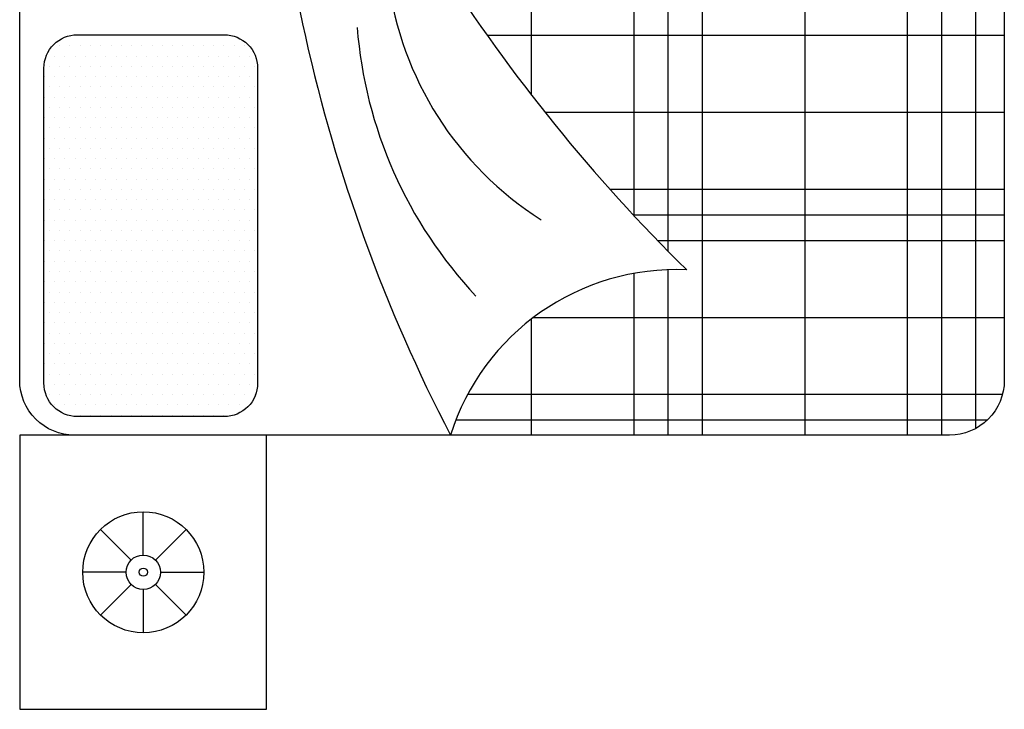
# Model space of a CAD drawing. Units: inches. Extents: x 528 to 2520, y -151 to 1354.
# Tile 32 of 41: x 2171 to 2226, y 731 to 770. Entities that reach past the tile are written whole.
import ezdxf

# ---------------------------------------------------------------- set-up
doc = ezdxf.new("R2010")
doc.units = ezdxf.units.IN
doc.header["$MEASUREMENT"] = 0
doc.layers.add('A-FURN', color=8, linetype='Continuous', lineweight=18)
doc.layers.add('BLOCK', color=6, linetype='Continuous')

# ---------------------------------------------------------------- blocks, each defined once
blk = doc.blocks.new('*X15')
at = {"color": 0}
for p, q in [((276.598, 451.25), (280.51, 451.25)), ((275.455, 450.625), (280.51, 450.625)), ((274.411, 450), (280.51, 450)), ((265.51, 448.125), (267.634, 448.125)), ((271.723, 448.125), (280.51, 448.125)), ((265.51, 446.25), (268.465, 446.25)), ((269.519, 446.25), (280.51, 446.25)), ((265.51, 445.625), (268.531, 445.625)), ((268.866, 445.625), (280.51, 445.625)), ((265.51, 445), (280.51, 445)), ((265.51, 443.125), (280.51, 443.125)), ((265.51, 441.25), (280.51, 441.25)), ((265.51, 440.625), (280.51, 440.625)), ((265.634, 440), (280.386, 440))]:
    blk.add_line(p, q, dxfattribs=at)
blk = doc.blocks.new('*X16')
at = {"color": 0}
for p, q in [((280.312, 439.886), (280.312, 452.896)), ((278.906, 439.482), (278.906, 452.338)), ((277.5, 439.482), (277.5, 451.702)), ((277.031, 439.482), (277.031, 451.471)), ((276.562, 439.482), (276.562, 451.231)), ((275.156, 439.482), (275.156, 450.451)), ((265.781, 439.797), (265.781, 449.511)), ((273.75, 439.482), (273.75, 449.576)), ((266.25, 439.517), (266.25, 449.296)), ((273.281, 439.482), (273.281, 449.261)), ((272.812, 439.482), (272.812, 448.934)), ((267.656, 439.482), (267.656, 448.095)), ((271.406, 439.482), (271.406, 447.876)), ((270, 439.482), (270, 446.689)), ((269.531, 439.482), (269.531, 446.262)), ((269.062, 439.482), (269.062, 445.817))]:
    blk.add_line(p, q, dxfattribs=at)
blk = doc.blocks.new('*X17')
at = {"color": 0}
for p, q in [((266.4375, 457.03125), (266.4375, 457.03125)), ((266.8125, 457.03125), (266.8125, 457.03125)), ((267.1875, 457.03125), (267.1875, 457.03125)), ((267.5625, 457.03125), (267.5625, 457.03125)), ((267.9375, 457.03125), (267.9375, 457.03125)), ((268.3125, 457.03125), (268.3125, 457.03125)), ((268.6875, 457.03125), (268.6875, 457.03125)), ((269.0625, 457.03125), (269.0625, 457.03125)), ((269.4375, 457.03125), (269.4375, 457.03125)), ((269.8125, 457.03125), (269.8125, 457.03125)), ((270.1875, 457.03125), (270.1875, 457.03125)), ((270.5625, 457.03125), (270.5625, 457.03125)), ((270.9375, 457.03125), (270.9375, 457.03125)), ((271.3125, 457.03125), (271.3125, 457.03125)), ((271.6875, 457.03125), (271.6875, 457.03125)), ((272.0625, 457.03125), (272.0625, 457.03125)), ((266.0625, 456.84375), (266.0625, 456.84375)), ((266.25, 456.9375), (266.25, 456.9375)), ((266.4375, 456.84375), (266.4375, 456.84375)), ((266.625, 456.9375), (266.625, 456.9375)), ((266.8125, 456.84375), (266.8125, 456.84375)), ((267, 456.9375), (267, 456.9375)), ((267.1875, 456.84375), (267.1875, 456.84375)), ((267.375, 456.9375), (267.375, 456.9375)), ((267.5625, 456.84375), (267.5625, 456.84375)), ((267.75, 456.9375), (267.75, 456.9375)), ((267.9375, 456.84375), (267.9375, 456.84375)), ((268.125, 456.9375), (268.125, 456.9375)), ((268.3125, 456.84375), (268.3125, 456.84375)), ((268.5, 456.9375), (268.5, 456.9375)), ((268.6875, 456.84375), (268.6875, 456.84375)), ((268.875, 456.9375), (268.875, 456.9375)), ((269.0625, 456.84375), (269.0625, 456.84375)), ((269.25, 456.9375), (269.25, 456.9375)), ((269.4375, 456.84375), (269.4375, 456.84375)), ((269.625, 456.9375), (269.625, 456.9375)), ((269.8125, 456.84375), (269.8125, 456.84375)), ((270, 456.9375), (270, 456.9375)), ((270.1875, 456.84375), (270.1875, 456.84375)), ((270.375, 456.9375), (270.375, 456.9375)), ((270.5625, 456.84375), (270.5625, 456.84375)), ((270.75, 456.9375), (270.75, 456.9375)), ((270.9375, 456.84375), (270.9375, 456.84375)), ((271.125, 456.9375), (271.125, 456.9375)), ((271.3125, 456.84375), (271.3125, 456.84375)), ((271.5, 456.9375), (271.5, 456.9375)), ((271.6875, 456.84375), (271.6875, 456.84375)), ((271.875, 456.9375), (271.875, 456.9375)), ((272.0625, 456.84375), (272.0625, 456.84375)), ((272.25, 456.9375), (272.25, 456.9375)), ((272.4375, 456.84375), (272.4375, 456.84375)), ((266.25, 456.75), (266.25, 456.75)), ((266.625, 456.75), (266.625, 456.75)), ((267, 456.75), (267, 456.75)), ((267.375, 456.75), (267.375, 456.75)), ((267.75, 456.75), (267.75, 456.75)), ((268.125, 456.75), (268.125, 456.75)), ((268.5, 456.75), (268.5, 456.75)), ((268.875, 456.75), (268.875, 456.75)), ((269.25, 456.75), (269.25, 456.75)), ((269.625, 456.75), (269.625, 456.75)), ((270, 456.75), (270, 456.75)), ((270.375, 456.75), (270.375, 456.75)), ((270.75, 456.75), (270.75, 456.75)), ((271.125, 456.75), (271.125, 456.75)), ((271.5, 456.75), (271.5, 456.75)), ((271.875, 456.75), (271.875, 456.75)), ((272.25, 456.75), (272.25, 456.75)), ((272.625, 456.75), (272.625, 456.75)), ((265.875, 456.5625), (265.875, 456.5625)), ((266.0625, 456.65625), (266.0625, 456.65625)), ((266.25, 456.5625), (266.25, 456.5625)), ((266.4375, 456.65625), (266.4375, 456.65625)), ((266.625, 456.5625), (266.625, 456.5625)), ((266.8125, 456.65625), (266.8125, 456.65625)), ((267, 456.5625), (267, 456.5625)), ((267.1875, 456.65625), (267.1875, 456.65625)), ((267.375, 456.5625), (267.375, 456.5625)), ((267.5625, 456.65625), (267.5625, 456.65625)), ((267.75, 456.5625), (267.75, 456.5625)), ((267.9375, 456.65625), (267.9375, 456.65625)), ((268.125, 456.5625), (268.125, 456.5625)), ((268.3125, 456.65625), (268.3125, 456.65625)), ((268.5, 456.5625), (268.5, 456.5625)), ((268.6875, 456.65625), (268.6875, 456.65625)), ((268.875, 456.5625), (268.875, 456.5625)), ((269.0625, 456.65625), (269.0625, 456.65625)), ((269.25, 456.5625), (269.25, 456.5625)), ((269.4375, 456.65625), (269.4375, 456.65625)), ((269.625, 456.5625), (269.625, 456.5625)), ((269.8125, 456.65625), (269.8125, 456.65625)), ((270, 456.5625), (270, 456.5625)), ((270.1875, 456.65625), (270.1875, 456.65625)), ((270.375, 456.5625), (270.375, 456.5625)), ((270.5625, 456.65625), (270.5625, 456.65625)), ((270.75, 456.5625), (270.75, 456.5625)), ((270.9375, 456.65625), (270.9375, 456.65625)), ((271.125, 456.5625), (271.125, 456.5625)), ((271.3125, 456.65625), (271.3125, 456.65625)), ((271.5, 456.5625), (271.5, 456.5625)), ((271.6875, 456.65625), (271.6875, 456.65625)), ((271.875, 456.5625), (271.875, 456.5625)), ((272.0625, 456.65625), (272.0625, 456.65625)), ((272.25, 456.5625), (272.25, 456.5625)), ((272.4375, 456.65625), (272.4375, 456.65625)), ((272.625, 456.5625), (272.625, 456.5625)), ((265.875, 456.375), (265.875, 456.375)), ((266.0625, 456.46875), (266.0625, 456.46875)), ((266.25, 456.375), (266.25, 456.375)), ((266.4375, 456.46875), (266.4375, 456.46875)), ((266.625, 456.375), (266.625, 456.375)), ((266.8125, 456.46875), (266.8125, 456.46875)), ((267, 456.375), (267, 456.375)), ((267.1875, 456.46875), (267.1875, 456.46875)), ((267.375, 456.375), (267.375, 456.375)), ((267.5625, 456.46875), (267.5625, 456.46875)), ((267.75, 456.375), (267.75, 456.375)), ((267.9375, 456.46875), (267.9375, 456.46875)), ((268.125, 456.375), (268.125, 456.375)), ((268.3125, 456.46875), (268.3125, 456.46875)), ((268.5, 456.375), (268.5, 456.375)), ((268.6875, 456.46875), (268.6875, 456.46875)), ((268.875, 456.375), (268.875, 456.375)), ((269.0625, 456.46875), (269.0625, 456.46875)), ((269.25, 456.375), (269.25, 456.375)), ((269.4375, 456.46875), (269.4375, 456.46875)), ((269.625, 456.375), (269.625, 456.375)), ((269.8125, 456.46875), (269.8125, 456.46875)), ((270, 456.375), (270, 456.375)), ((270.1875, 456.46875), (270.1875, 456.46875)), ((270.375, 456.375), (270.375, 456.375)), ((270.5625, 456.46875), (270.5625, 456.46875)), ((270.75, 456.375), (270.75, 456.375)), ((270.9375, 456.46875), (270.9375, 456.46875)), ((271.125, 456.375), (271.125, 456.375)), ((271.3125, 456.46875), (271.3125, 456.46875)), ((271.5, 456.375), (271.5, 456.375)), ((271.6875, 456.46875), (271.6875, 456.46875)), ((271.875, 456.375), (271.875, 456.375)), ((272.0625, 456.46875), (272.0625, 456.46875)), ((272.25, 456.375), (272.25, 456.375)), ((272.4375, 456.46875), (272.4375, 456.46875)), ((272.625, 456.375), (272.625, 456.375)), ((272.8125, 456.46875), (272.8125, 456.46875)), ((265.875, 456.1875), (265.875, 456.1875)), ((266.0625, 456.28125), (266.0625, 456.28125)), ((266.25, 456.1875), (266.25, 456.1875)), ((266.4375, 456.28125), (266.4375, 456.28125)), ((266.625, 456.1875), (266.625, 456.1875)), ((266.8125, 456.28125), (266.8125, 456.28125)), ((267, 456.1875), (267, 456.1875)), ((267.1875, 456.28125), (267.1875, 456.28125)), ((267.375, 456.1875), (267.375, 456.1875)), ((267.5625, 456.28125), (267.5625, 456.28125)), ((267.75, 456.1875), (267.75, 456.1875)), ((267.9375, 456.28125), (267.9375, 456.28125)), ((268.125, 456.1875), (268.125, 456.1875)), ((268.3125, 456.28125), (268.3125, 456.28125)), ((268.5, 456.1875), (268.5, 456.1875)), ((268.6875, 456.28125), (268.6875, 456.28125)), ((268.875, 456.1875), (268.875, 456.1875)), ((269.0625, 456.28125), (269.0625, 456.28125)), ((269.25, 456.1875), (269.25, 456.1875)), ((269.4375, 456.28125), (269.4375, 456.28125)), ((269.625, 456.1875), (269.625, 456.1875)), ((269.8125, 456.28125), (269.8125, 456.28125)), ((270, 456.1875), (270, 456.1875)), ((270.1875, 456.28125), (270.1875, 456.28125)), ((270.375, 456.1875), (270.375, 456.1875)), ((270.5625, 456.28125), (270.5625, 456.28125)), ((270.75, 456.1875), (270.75, 456.1875)), ((270.9375, 456.28125), (270.9375, 456.28125)), ((271.125, 456.1875), (271.125, 456.1875)), ((271.3125, 456.28125), (271.3125, 456.28125)), ((271.5, 456.1875), (271.5, 456.1875)), ((271.6875, 456.28125), (271.6875, 456.28125)), ((271.875, 456.1875), (271.875, 456.1875)), ((272.0625, 456.28125), (272.0625, 456.28125)), ((272.25, 456.1875), (272.25, 456.1875)), ((272.4375, 456.28125), (272.4375, 456.28125)), ((272.625, 456.1875), (272.625, 456.1875)), ((272.8125, 456.28125), (272.8125, 456.28125)), ((265.875, 456), (265.875, 456)), ((266.0625, 456.09375), (266.0625, 456.09375)), ((266.25, 456), (266.25, 456)), ((266.4375, 456.09375), (266.4375, 456.09375)), ((266.625, 456), (266.625, 456)), ((266.8125, 456.09375), (266.8125, 456.09375)), ((267, 456), (267, 456)), ((267.1875, 456.09375), (267.1875, 456.09375)), ((267.375, 456), (267.375, 456)), ((267.5625, 456.09375), (267.5625, 456.09375)), ((267.75, 456), (267.75, 456)), ((267.9375, 456.09375), (267.9375, 456.09375)), ((268.125, 456), (268.125, 456)), ((268.3125, 456.09375), (268.3125, 456.09375)), ((268.5, 456), (268.5, 456)), ((268.6875, 456.09375), (268.6875, 456.09375)), ((268.875, 456), (268.875, 456)), ((269.0625, 456.09375), (269.0625, 456.09375)), ((269.25, 456), (269.25, 456)), ((269.4375, 456.09375), (269.4375, 456.09375)), ((269.625, 456), (269.625, 456)), ((269.8125, 456.09375), (269.8125, 456.09375)), ((270, 456), (270, 456)), ((270.1875, 456.09375), (270.1875, 456.09375)), ((270.375, 456), (270.375, 456)), ((270.5625, 456.09375), (270.5625, 456.09375)), ((270.75, 456), (270.75, 456)), ((270.9375, 456.09375), (270.9375, 456.09375)), ((271.125, 456), (271.125, 456)), ((271.3125, 456.09375), (271.3125, 456.09375)), ((271.5, 456), (271.5, 456)), ((271.6875, 456.09375), (271.6875, 456.09375)), ((271.875, 456), (271.875, 456)), ((272.0625, 456.09375), (272.0625, 456.09375)), ((272.25, 456), (272.25, 456)), ((272.4375, 456.09375), (272.4375, 456.09375)), ((272.625, 456), (272.625, 456)), ((272.8125, 456.09375), (272.8125, 456.09375)), ((265.875, 455.8125), (265.875, 455.8125)), ((266.0625, 455.90625), (266.0625, 455.90625)), ((266.25, 455.8125), (266.25, 455.8125)), ((266.4375, 455.90625), (266.4375, 455.90625)), ((266.625, 455.8125), (266.625, 455.8125)), ((266.8125, 455.90625), (266.8125, 455.90625)), ((267, 455.8125), (267, 455.8125)), ((267.1875, 455.90625), (267.1875, 455.90625)), ((267.375, 455.8125), (267.375, 455.8125)), ((267.5625, 455.90625), (267.5625, 455.90625)), ((267.75, 455.8125), (267.75, 455.8125)), ((267.9375, 455.90625), (267.9375, 455.90625)), ((268.125, 455.8125), (268.125, 455.8125)), ((268.3125, 455.90625), (268.3125, 455.90625)), ((268.5, 455.8125), (268.5, 455.8125)), ((268.6875, 455.90625), (268.6875, 455.90625)), ((268.875, 455.8125), (268.875, 455.8125)), ((269.0625, 455.90625), (269.0625, 455.90625)), ((269.25, 455.8125), (269.25, 455.8125)), ((269.4375, 455.90625), (269.4375, 455.90625)), ((269.625, 455.8125), (269.625, 455.8125)), ((269.8125, 455.90625), (269.8125, 455.90625)), ((270, 455.8125), (270, 455.8125)), ((270.1875, 455.90625), (270.1875, 455.90625)), ((270.375, 455.8125), (270.375, 455.8125)), ((270.5625, 455.90625), (270.5625, 455.90625)), ((270.75, 455.8125), (270.75, 455.8125)), ((270.9375, 455.90625), (270.9375, 455.90625)), ((271.125, 455.8125), (271.125, 455.8125)), ((271.3125, 455.90625), (271.3125, 455.90625)), ((271.5, 455.8125), (271.5, 455.8125)), ((271.6875, 455.90625), (271.6875, 455.90625)), ((271.875, 455.8125), (271.875, 455.8125)), ((272.0625, 455.90625), (272.0625, 455.90625)), ((272.25, 455.8125), (272.25, 455.8125)), ((272.4375, 455.90625), (272.4375, 455.90625)), ((272.625, 455.8125), (272.625, 455.8125)), ((272.8125, 455.90625), (272.8125, 455.90625)), ((265.875, 455.625), (265.875, 455.625)), ((266.0625, 455.71875), (266.0625, 455.71875)), ((266.25, 455.625), (266.25, 455.625)), ((266.4375, 455.71875), (266.4375, 455.71875)), ((266.625, 455.625), (266.625, 455.625)), ((266.8125, 455.71875), (266.8125, 455.71875)), ((267, 455.625), (267, 455.625)), ((267.1875, 455.71875), (267.1875, 455.71875)), ((267.375, 455.625), (267.375, 455.625)), ((267.5625, 455.71875), (267.5625, 455.71875)), ((267.75, 455.625), (267.75, 455.625)), ((267.9375, 455.71875), (267.9375, 455.71875)), ((268.125, 455.625), (268.125, 455.625)), ((268.3125, 455.71875), (268.3125, 455.71875)), ((268.5, 455.625), (268.5, 455.625)), ((268.6875, 455.71875), (268.6875, 455.71875)), ((268.875, 455.625), (268.875, 455.625)), ((269.0625, 455.71875), (269.0625, 455.71875)), ((269.25, 455.625), (269.25, 455.625)), ((269.4375, 455.71875), (269.4375, 455.71875)), ((269.625, 455.625), (269.625, 455.625)), ((269.8125, 455.71875), (269.8125, 455.71875)), ((270, 455.625), (270, 455.625)), ((270.1875, 455.71875), (270.1875, 455.71875)), ((270.375, 455.625), (270.375, 455.625)), ((270.5625, 455.71875), (270.5625, 455.71875)), ((270.75, 455.625), (270.75, 455.625)), ((270.9375, 455.71875), (270.9375, 455.71875)), ((271.125, 455.625), (271.125, 455.625)), ((271.3125, 455.71875), (271.3125, 455.71875)), ((271.5, 455.625), (271.5, 455.625)), ((271.6875, 455.71875), (271.6875, 455.71875)), ((271.875, 455.625), (271.875, 455.625)), ((272.0625, 455.71875), (272.0625, 455.71875)), ((272.25, 455.625), (272.25, 455.625)), ((272.4375, 455.71875), (272.4375, 455.71875)), ((272.625, 455.625), (272.625, 455.625)), ((272.8125, 455.71875), (272.8125, 455.71875)), ((265.875, 455.4375), (265.875, 455.4375)), ((266.0625, 455.53125), (266.0625, 455.53125)), ((266.25, 455.4375), (266.25, 455.4375)), ((266.4375, 455.53125), (266.4375, 455.53125)), ((266.625, 455.4375), (266.625, 455.4375)), ((266.8125, 455.53125), (266.8125, 455.53125)), ((267, 455.4375), (267, 455.4375)), ((267.1875, 455.53125), (267.1875, 455.53125)), ((267.375, 455.4375), (267.375, 455.4375)), ((267.5625, 455.53125), (267.5625, 455.53125)), ((267.75, 455.4375), (267.75, 455.4375)), ((267.9375, 455.53125), (267.9375, 455.53125)), ((268.125, 455.4375), (268.125, 455.4375)), ((268.3125, 455.53125), (268.3125, 455.53125)), ((268.5, 455.4375), (268.5, 455.4375)), ((268.6875, 455.53125), (268.6875, 455.53125)), ((268.875, 455.4375), (268.875, 455.4375)), ((269.0625, 455.53125), (269.0625, 455.53125)), ((269.25, 455.4375), (269.25, 455.4375)), ((269.4375, 455.53125), (269.4375, 455.53125)), ((269.625, 455.4375), (269.625, 455.4375)), ((269.8125, 455.53125), (269.8125, 455.53125)), ((270, 455.4375), (270, 455.4375)), ((270.1875, 455.53125), (270.1875, 455.53125)), ((270.375, 455.4375), (270.375, 455.4375)), ((270.5625, 455.53125), (270.5625, 455.53125)), ((270.75, 455.4375), (270.75, 455.4375)), ((270.9375, 455.53125), (270.9375, 455.53125)), ((271.125, 455.4375), (271.125, 455.4375)), ((271.3125, 455.53125), (271.3125, 455.53125)), ((271.5, 455.4375), (271.5, 455.4375)), ((271.6875, 455.53125), (271.6875, 455.53125)), ((271.875, 455.4375), (271.875, 455.4375)), ((272.0625, 455.53125), (272.0625, 455.53125)), ((272.25, 455.4375), (272.25, 455.4375)), ((272.4375, 455.53125), (272.4375, 455.53125)), ((272.625, 455.4375), (272.625, 455.4375)), ((272.8125, 455.53125), (272.8125, 455.53125)), ((265.875, 455.25), (265.875, 455.25)), ((266.0625, 455.34375), (266.0625, 455.34375)), ((266.25, 455.25), (266.25, 455.25)), ((266.4375, 455.34375), (266.4375, 455.34375)), ((266.625, 455.25), (266.625, 455.25)), ((266.8125, 455.34375), (266.8125, 455.34375)), ((267, 455.25), (267, 455.25)), ((267.1875, 455.34375), (267.1875, 455.34375)), ((267.375, 455.25), (267.375, 455.25)), ((267.5625, 455.34375), (267.5625, 455.34375)), ((267.75, 455.25), (267.75, 455.25)), ((267.9375, 455.34375), (267.9375, 455.34375)), ((268.125, 455.25), (268.125, 455.25)), ((268.3125, 455.34375), (268.3125, 455.34375)), ((268.5, 455.25), (268.5, 455.25)), ((268.6875, 455.34375), (268.6875, 455.34375)), ((268.875, 455.25), (268.875, 455.25)), ((269.0625, 455.34375), (269.0625, 455.34375)), ((269.25, 455.25), (269.25, 455.25)), ((269.4375, 455.34375), (269.4375, 455.34375)), ((269.625, 455.25), (269.625, 455.25)), ((269.8125, 455.34375), (269.8125, 455.34375)), ((270, 455.25), (270, 455.25)), ((270.1875, 455.34375), (270.1875, 455.34375)), ((270.375, 455.25), (270.375, 455.25)), ((270.5625, 455.34375), (270.5625, 455.34375)), ((270.75, 455.25), (270.75, 455.25)), ((270.9375, 455.34375), (270.9375, 455.34375)), ((271.125, 455.25), (271.125, 455.25)), ((271.3125, 455.34375), (271.3125, 455.34375)), ((271.5, 455.25), (271.5, 455.25)), ((271.6875, 455.34375), (271.6875, 455.34375)), ((271.875, 455.25), (271.875, 455.25)), ((272.0625, 455.34375), (272.0625, 455.34375)), ((272.25, 455.25), (272.25, 455.25)), ((272.4375, 455.34375), (272.4375, 455.34375)), ((272.625, 455.25), (272.625, 455.25)), ((272.8125, 455.34375), (272.8125, 455.34375)), ((265.875, 455.0625), (265.875, 455.0625)), ((266.0625, 455.15625), (266.0625, 455.15625)), ((266.25, 455.0625), (266.25, 455.0625)), ((266.4375, 455.15625), (266.4375, 455.15625)), ((266.625, 455.0625), (266.625, 455.0625)), ((266.8125, 455.15625), (266.8125, 455.15625)), ((267, 455.0625), (267, 455.0625)), ((267.1875, 455.15625), (267.1875, 455.15625)), ((267.375, 455.0625), (267.375, 455.0625)), ((267.5625, 455.15625), (267.5625, 455.15625)), ((267.75, 455.0625), (267.75, 455.0625)), ((267.9375, 455.15625), (267.9375, 455.15625)), ((268.125, 455.0625), (268.125, 455.0625)), ((268.3125, 455.15625), (268.3125, 455.15625)), ((268.5, 455.0625), (268.5, 455.0625)), ((268.6875, 455.15625), (268.6875, 455.15625)), ((268.875, 455.0625), (268.875, 455.0625)), ((269.0625, 455.15625), (269.0625, 455.15625)), ((269.25, 455.0625), (269.25, 455.0625)), ((269.4375, 455.15625), (269.4375, 455.15625)), ((269.625, 455.0625), (269.625, 455.0625)), ((269.8125, 455.15625), (269.8125, 455.15625)), ((270, 455.0625), (270, 455.0625)), ((270.1875, 455.15625), (270.1875, 455.15625)), ((270.375, 455.0625), (270.375, 455.0625)), ((270.5625, 455.15625), (270.5625, 455.15625)), ((270.75, 455.0625), (270.75, 455.0625)), ((270.9375, 455.15625), (270.9375, 455.15625)), ((271.125, 455.0625), (271.125, 455.0625)), ((271.3125, 455.15625), (271.3125, 455.15625)), ((271.5, 455.0625), (271.5, 455.0625)), ((271.6875, 455.15625), (271.6875, 455.15625)), ((271.875, 455.0625), (271.875, 455.0625)), ((272.0625, 455.15625), (272.0625, 455.15625)), ((272.25, 455.0625), (272.25, 455.0625)), ((272.4375, 455.15625), (272.4375, 455.15625)), ((272.625, 455.0625), (272.625, 455.0625)), ((272.8125, 455.15625), (272.8125, 455.15625)), ((265.875, 454.875), (265.875, 454.875)), ((266.0625, 454.96875), (266.0625, 454.96875)), ((266.25, 454.875), (266.25, 454.875)), ((266.4375, 454.96875), (266.4375, 454.96875)), ((266.625, 454.875), (266.625, 454.875)), ((266.8125, 454.96875), (266.8125, 454.96875)), ((267, 454.875), (267, 454.875)), ((267.1875, 454.96875), (267.1875, 454.96875)), ((267.375, 454.875), (267.375, 454.875)), ((267.5625, 454.96875), (267.5625, 454.96875)), ((267.75, 454.875), (267.75, 454.875)), ((267.9375, 454.96875), (267.9375, 454.96875)), ((268.125, 454.875), (268.125, 454.875)), ((268.3125, 454.96875), (268.3125, 454.96875)), ((268.5, 454.875), (268.5, 454.875)), ((268.6875, 454.96875), (268.6875, 454.96875)), ((268.875, 454.875), (268.875, 454.875)), ((269.0625, 454.96875), (269.0625, 454.96875)), ((269.25, 454.875), (269.25, 454.875)), ((269.4375, 454.96875), (269.4375, 454.96875)), ((269.625, 454.875), (269.625, 454.875)), ((269.8125, 454.96875), (269.8125, 454.96875)), ((270, 454.875), (270, 454.875)), ((270.1875, 454.96875), (270.1875, 454.96875)), ((270.375, 454.875), (270.375, 454.875)), ((270.5625, 454.96875), (270.5625, 454.96875)), ((270.75, 454.875), (270.75, 454.875)), ((270.9375, 454.96875), (270.9375, 454.96875)), ((271.125, 454.875), (271.125, 454.875)), ((271.3125, 454.96875), (271.3125, 454.96875)), ((271.5, 454.875), (271.5, 454.875)), ((271.6875, 454.96875), (271.6875, 454.96875)), ((271.875, 454.875), (271.875, 454.875)), ((272.0625, 454.96875), (272.0625, 454.96875)), ((272.25, 454.875), (272.25, 454.875)), ((272.4375, 454.96875), (272.4375, 454.96875)), ((272.625, 454.875), (272.625, 454.875)), ((272.8125, 454.96875), (272.8125, 454.96875)), ((265.875, 454.6875), (265.875, 454.6875)), ((266.0625, 454.78125), (266.0625, 454.78125)), ((266.25, 454.6875), (266.25, 454.6875)), ((266.4375, 454.78125), (266.4375, 454.78125)), ((266.625, 454.6875), (266.625, 454.6875)), ((266.8125, 454.78125), (266.8125, 454.78125)), ((267, 454.6875), (267, 454.6875)), ((267.1875, 454.78125), (267.1875, 454.78125)), ((267.375, 454.6875), (267.375, 454.6875)), ((267.5625, 454.78125), (267.5625, 454.78125)), ((267.75, 454.6875), (267.75, 454.6875)), ((267.9375, 454.78125), (267.9375, 454.78125)), ((268.125, 454.6875), (268.125, 454.6875)), ((268.3125, 454.78125), (268.3125, 454.78125)), ((268.5, 454.6875), (268.5, 454.6875)), ((268.6875, 454.78125), (268.6875, 454.78125)), ((268.875, 454.6875), (268.875, 454.6875)), ((269.0625, 454.78125), (269.0625, 454.78125)), ((269.25, 454.6875), (269.25, 454.6875)), ((269.4375, 454.78125), (269.4375, 454.78125)), ((269.625, 454.6875), (269.625, 454.6875)), ((269.8125, 454.78125), (269.8125, 454.78125)), ((270, 454.6875), (270, 454.6875)), ((270.1875, 454.78125), (270.1875, 454.78125)), ((270.375, 454.6875), (270.375, 454.6875)), ((270.5625, 454.78125), (270.5625, 454.78125)), ((270.75, 454.6875), (270.75, 454.6875)), ((270.9375, 454.78125), (270.9375, 454.78125)), ((271.125, 454.6875), (271.125, 454.6875)), ((271.3125, 454.78125), (271.3125, 454.78125)), ((271.5, 454.6875), (271.5, 454.6875)), ((271.6875, 454.78125), (271.6875, 454.78125)), ((271.875, 454.6875), (271.875, 454.6875)), ((272.0625, 454.78125), (272.0625, 454.78125)), ((272.25, 454.6875), (272.25, 454.6875)), ((272.4375, 454.78125), (272.4375, 454.78125)), ((272.625, 454.6875), (272.625, 454.6875)), ((272.8125, 454.78125), (272.8125, 454.78125)), ((266.0625, 454.59375), (266.0625, 454.59375)), ((266.4375, 454.59375), (266.4375, 454.59375)), ((266.8125, 454.59375), (266.8125, 454.59375)), ((267.1875, 454.59375), (267.1875, 454.59375)), ((267.5625, 454.59375), (267.5625, 454.59375)), ((267.9375, 454.59375), (267.9375, 454.59375)), ((268.3125, 454.59375), (268.3125, 454.59375)), ((268.6875, 454.59375), (268.6875, 454.59375)), ((269.0625, 454.59375), (269.0625, 454.59375)), ((269.4375, 454.59375), (269.4375, 454.59375)), ((269.8125, 454.59375), (269.8125, 454.59375)), ((270.1875, 454.59375), (270.1875, 454.59375)), ((270.5625, 454.59375), (270.5625, 454.59375)), ((270.9375, 454.59375), (270.9375, 454.59375)), ((271.3125, 454.59375), (271.3125, 454.59375)), ((271.6875, 454.59375), (271.6875, 454.59375)), ((272.0625, 454.59375), (272.0625, 454.59375)), ((272.4375, 454.59375), (272.4375, 454.59375)), ((272.8125, 454.59375), (272.8125, 454.59375)), ((265.875, 454.5), (265.875, 454.5)), ((266.0625, 454.40625), (266.0625, 454.40625)), ((266.25, 454.5), (266.25, 454.5)), ((266.4375, 454.40625), (266.4375, 454.40625)), ((266.625, 454.5), (266.625, 454.5)), ((266.8125, 454.40625), (266.8125, 454.40625)), ((267, 454.5), (267, 454.5)), ((267.1875, 454.40625), (267.1875, 454.40625)), ((267.375, 454.5), (267.375, 454.5)), ((267.5625, 454.40625), (267.5625, 454.40625)), ((267.75, 454.5), (267.75, 454.5)), ((267.9375, 454.40625), (267.9375, 454.40625)), ((268.125, 454.5), (268.125, 454.5)), ((268.3125, 454.40625), (268.3125, 454.40625)), ((268.5, 454.5), (268.5, 454.5)), ((268.6875, 454.40625), (268.6875, 454.40625)), ((268.875, 454.5), (268.875, 454.5)), ((269.0625, 454.40625), (269.0625, 454.40625)), ((269.25, 454.5), (269.25, 454.5)), ((269.4375, 454.40625), (269.4375, 454.40625)), ((269.625, 454.5), (269.625, 454.5)), ((269.8125, 454.40625), (269.8125, 454.40625)), ((270, 454.5), (270, 454.5)), ((270.1875, 454.40625), (270.1875, 454.40625)), ((270.375, 454.5), (270.375, 454.5)), ((270.5625, 454.40625), (270.5625, 454.40625)), ((270.75, 454.5), (270.75, 454.5)), ((270.9375, 454.40625), (270.9375, 454.40625)), ((271.125, 454.5), (271.125, 454.5)), ((271.3125, 454.40625), (271.3125, 454.40625)), ((271.5, 454.5), (271.5, 454.5)), ((271.6875, 454.40625), (271.6875, 454.40625)), ((271.875, 454.5), (271.875, 454.5)), ((272.0625, 454.40625), (272.0625, 454.40625)), ((272.25, 454.5), (272.25, 454.5)), ((272.4375, 454.40625), (272.4375, 454.40625)), ((272.625, 454.5), (272.625, 454.5)), ((272.8125, 454.40625), (272.8125, 454.40625)), ((265.875, 454.3125), (265.875, 454.3125)), ((266.0625, 454.21875), (266.0625, 454.21875)), ((266.25, 454.3125), (266.25, 454.3125)), ((266.4375, 454.21875), (266.4375, 454.21875)), ((266.625, 454.3125), (266.625, 454.3125)), ((266.8125, 454.21875), (266.8125, 454.21875)), ((267, 454.3125), (267, 454.3125)), ((267.1875, 454.21875), (267.1875, 454.21875)), ((267.375, 454.3125), (267.375, 454.3125)), ((267.5625, 454.21875), (267.5625, 454.21875)), ((267.75, 454.3125), (267.75, 454.3125)), ((267.9375, 454.21875), (267.9375, 454.21875)), ((268.125, 454.3125), (268.125, 454.3125)), ((268.3125, 454.21875), (268.3125, 454.21875)), ((268.5, 454.3125), (268.5, 454.3125)), ((268.6875, 454.21875), (268.6875, 454.21875)), ((268.875, 454.3125), (268.875, 454.3125)), ((269.0625, 454.21875), (269.0625, 454.21875)), ((269.25, 454.3125), (269.25, 454.3125)), ((269.4375, 454.21875), (269.4375, 454.21875)), ((269.625, 454.3125), (269.625, 454.3125)), ((269.8125, 454.21875), (269.8125, 454.21875)), ((270, 454.3125), (270, 454.3125)), ((270.1875, 454.21875), (270.1875, 454.21875)), ((270.375, 454.3125), (270.375, 454.3125)), ((270.5625, 454.21875), (270.5625, 454.21875)), ((270.75, 454.3125), (270.75, 454.3125)), ((270.9375, 454.21875), (270.9375, 454.21875)), ((271.125, 454.3125), (271.125, 454.3125)), ((271.3125, 454.21875), (271.3125, 454.21875)), ((271.5, 454.3125), (271.5, 454.3125)), ((271.6875, 454.21875), (271.6875, 454.21875)), ((271.875, 454.3125), (271.875, 454.3125)), ((272.0625, 454.21875), (272.0625, 454.21875)), ((272.25, 454.3125), (272.25, 454.3125)), ((272.4375, 454.21875), (272.4375, 454.21875)), ((272.625, 454.3125), (272.625, 454.3125)), ((272.8125, 454.21875), (272.8125, 454.21875)), ((265.875, 454.125), (265.875, 454.125)), ((266.0625, 454.03125), (266.0625, 454.03125)), ((266.25, 454.125), (266.25, 454.125)), ((266.4375, 454.03125), (266.4375, 454.03125)), ((266.625, 454.125), (266.625, 454.125)), ((266.8125, 454.03125), (266.8125, 454.03125)), ((267, 454.125), (267, 454.125)), ((267.1875, 454.03125), (267.1875, 454.03125)), ((267.375, 454.125), (267.375, 454.125)), ((267.5625, 454.03125), (267.5625, 454.03125)), ((267.75, 454.125), (267.75, 454.125)), ((267.9375, 454.03125), (267.9375, 454.03125)), ((268.125, 454.125), (268.125, 454.125)), ((268.3125, 454.03125), (268.3125, 454.03125)), ((268.5, 454.125), (268.5, 454.125)), ((268.6875, 454.03125), (268.6875, 454.03125)), ((268.875, 454.125), (268.875, 454.125)), ((269.0625, 454.03125), (269.0625, 454.03125)), ((269.25, 454.125), (269.25, 454.125)), ((269.4375, 454.03125), (269.4375, 454.03125)), ((269.625, 454.125), (269.625, 454.125)), ((269.8125, 454.03125), (269.8125, 454.03125)), ((270, 454.125), (270, 454.125)), ((270.1875, 454.03125), (270.1875, 454.03125)), ((270.375, 454.125), (270.375, 454.125)), ((270.5625, 454.03125), (270.5625, 454.03125)), ((270.75, 454.125), (270.75, 454.125)), ((270.9375, 454.03125), (270.9375, 454.03125)), ((271.125, 454.125), (271.125, 454.125)), ((271.3125, 454.03125), (271.3125, 454.03125)), ((271.5, 454.125), (271.5, 454.125)), ((271.6875, 454.03125), (271.6875, 454.03125)), ((271.875, 454.125), (271.875, 454.125)), ((272.0625, 454.03125), (272.0625, 454.03125)), ((272.25, 454.125), (272.25, 454.125)), ((272.4375, 454.03125), (272.4375, 454.03125)), ((272.625, 454.125), (272.625, 454.125)), ((272.8125, 454.03125), (272.8125, 454.03125)), ((265.875, 453.9375), (265.875, 453.9375)), ((266.0625, 453.84375), (266.0625, 453.84375)), ((266.25, 453.9375), (266.25, 453.9375)), ((266.4375, 453.84375), (266.4375, 453.84375)), ((266.625, 453.9375), (266.625, 453.9375)), ((266.8125, 453.84375), (266.8125, 453.84375)), ((267, 453.9375), (267, 453.9375)), ((267.1875, 453.84375), (267.1875, 453.84375)), ((267.375, 453.9375), (267.375, 453.9375)), ((267.5625, 453.84375), (267.5625, 453.84375)), ((267.75, 453.9375), (267.75, 453.9375)), ((267.9375, 453.84375), (267.9375, 453.84375)), ((268.125, 453.9375), (268.125, 453.9375)), ((268.3125, 453.84375), (268.3125, 453.84375)), ((268.5, 453.9375), (268.5, 453.9375)), ((268.6875, 453.84375), (268.6875, 453.84375)), ((268.875, 453.9375), (268.875, 453.9375)), ((269.0625, 453.84375), (269.0625, 453.84375)), ((269.25, 453.9375), (269.25, 453.9375)), ((269.4375, 453.84375), (269.4375, 453.84375)), ((269.625, 453.9375), (269.625, 453.9375)), ((269.8125, 453.84375), (269.8125, 453.84375)), ((270, 453.9375), (270, 453.9375)), ((270.1875, 453.84375), (270.1875, 453.84375)), ((270.375, 453.9375), (270.375, 453.9375)), ((270.5625, 453.84375), (270.5625, 453.84375)), ((270.75, 453.9375), (270.75, 453.9375)), ((270.9375, 453.84375), (270.9375, 453.84375)), ((271.125, 453.9375), (271.125, 453.9375)), ((271.3125, 453.84375), (271.3125, 453.84375)), ((271.5, 453.9375), (271.5, 453.9375)), ((271.6875, 453.84375), (271.6875, 453.84375)), ((271.875, 453.9375), (271.875, 453.9375)), ((272.0625, 453.84375), (272.0625, 453.84375)), ((272.25, 453.9375), (272.25, 453.9375)), ((272.4375, 453.84375), (272.4375, 453.84375)), ((272.625, 453.9375), (272.625, 453.9375)), ((272.8125, 453.84375), (272.8125, 453.84375)), ((265.875, 453.75), (265.875, 453.75)), ((266.0625, 453.65625), (266.0625, 453.65625)), ((266.25, 453.75), (266.25, 453.75)), ((266.4375, 453.65625), (266.4375, 453.65625)), ((266.625, 453.75), (266.625, 453.75)), ((266.8125, 453.65625), (266.8125, 453.65625)), ((267, 453.75), (267, 453.75)), ((267.1875, 453.65625), (267.1875, 453.65625)), ((267.375, 453.75), (267.375, 453.75)), ((267.5625, 453.65625), (267.5625, 453.65625)), ((267.75, 453.75), (267.75, 453.75)), ((267.9375, 453.65625), (267.9375, 453.65625)), ((268.125, 453.75), (268.125, 453.75)), ((268.3125, 453.65625), (268.3125, 453.65625)), ((268.5, 453.75), (268.5, 453.75)), ((268.6875, 453.65625), (268.6875, 453.65625)), ((268.875, 453.75), (268.875, 453.75)), ((269.0625, 453.65625), (269.0625, 453.65625)), ((269.25, 453.75), (269.25, 453.75)), ((269.4375, 453.65625), (269.4375, 453.65625)), ((269.625, 453.75), (269.625, 453.75)), ((269.8125, 453.65625), (269.8125, 453.65625)), ((270, 453.75), (270, 453.75)), ((270.1875, 453.65625), (270.1875, 453.65625)), ((270.375, 453.75), (270.375, 453.75)), ((270.5625, 453.65625), (270.5625, 453.65625)), ((270.75, 453.75), (270.75, 453.75)), ((270.9375, 453.65625), (270.9375, 453.65625)), ((271.125, 453.75), (271.125, 453.75)), ((271.3125, 453.65625), (271.3125, 453.65625)), ((271.5, 453.75), (271.5, 453.75)), ((271.6875, 453.65625), (271.6875, 453.65625)), ((271.875, 453.75), (271.875, 453.75)), ((272.0625, 453.65625), (272.0625, 453.65625)), ((272.25, 453.75), (272.25, 453.75)), ((272.4375, 453.65625), (272.4375, 453.65625)), ((272.625, 453.75), (272.625, 453.75)), ((272.8125, 453.65625), (272.8125, 453.65625)), ((266.0625, 453.46875), (266.0625, 453.46875)), ((266.25, 453.5625), (266.25, 453.5625)), ((266.4375, 453.46875), (266.4375, 453.46875)), ((266.625, 453.5625), (266.625, 453.5625)), ((266.8125, 453.46875), (266.8125, 453.46875)), ((267, 453.5625), (267, 453.5625)), ((267.1875, 453.46875), (267.1875, 453.46875)), ((267.375, 453.5625), (267.375, 453.5625)), ((267.5625, 453.46875), (267.5625, 453.46875)), ((267.75, 453.5625), (267.75, 453.5625)), ((267.9375, 453.46875), (267.9375, 453.46875)), ((268.125, 453.5625), (268.125, 453.5625)), ((268.3125, 453.46875), (268.3125, 453.46875)), ((268.5, 453.5625), (268.5, 453.5625)), ((268.6875, 453.46875), (268.6875, 453.46875)), ((268.875, 453.5625), (268.875, 453.5625)), ((269.0625, 453.46875), (269.0625, 453.46875)), ((269.25, 453.5625), (269.25, 453.5625)), ((269.4375, 453.46875), (269.4375, 453.46875)), ((269.625, 453.5625), (269.625, 453.5625)), ((269.8125, 453.46875), (269.8125, 453.46875)), ((270, 453.5625), (270, 453.5625)), ((270.1875, 453.46875), (270.1875, 453.46875)), ((270.375, 453.5625), (270.375, 453.5625)), ((270.5625, 453.46875), (270.5625, 453.46875)), ((270.75, 453.5625), (270.75, 453.5625)), ((270.9375, 453.46875), (270.9375, 453.46875)), ((271.125, 453.5625), (271.125, 453.5625)), ((271.3125, 453.46875), (271.3125, 453.46875)), ((271.5, 453.5625), (271.5, 453.5625)), ((271.6875, 453.46875), (271.6875, 453.46875)), ((271.875, 453.5625), (271.875, 453.5625)), ((272.0625, 453.46875), (272.0625, 453.46875)), ((272.25, 453.5625), (272.25, 453.5625)), ((272.4375, 453.46875), (272.4375, 453.46875)), ((272.625, 453.5625), (272.625, 453.5625)), ((266.0625, 453.28125), (266.0625, 453.28125)), ((266.25, 453.375), (266.25, 453.375)), ((266.4375, 453.28125), (266.4375, 453.28125)), ((266.625, 453.375), (266.625, 453.375)), ((266.8125, 453.28125), (266.8125, 453.28125)), ((267, 453.375), (267, 453.375)), ((267.1875, 453.28125), (267.1875, 453.28125)), ((267.375, 453.375), (267.375, 453.375)), ((267.5625, 453.28125), (267.5625, 453.28125)), ((267.75, 453.375), (267.75, 453.375)), ((267.9375, 453.28125), (267.9375, 453.28125)), ((268.125, 453.375), (268.125, 453.375)), ((268.3125, 453.28125), (268.3125, 453.28125)), ((268.5, 453.375), (268.5, 453.375)), ((268.6875, 453.28125), (268.6875, 453.28125)), ((268.875, 453.375), (268.875, 453.375)), ((269.0625, 453.28125), (269.0625, 453.28125)), ((269.25, 453.375), (269.25, 453.375)), ((269.4375, 453.28125), (269.4375, 453.28125)), ((269.625, 453.375), (269.625, 453.375)), ((269.8125, 453.28125), (269.8125, 453.28125)), ((270, 453.375), (270, 453.375)), ((270.1875, 453.28125), (270.1875, 453.28125)), ((270.375, 453.375), (270.375, 453.375)), ((270.5625, 453.28125), (270.5625, 453.28125)), ((270.75, 453.375), (270.75, 453.375)), ((270.9375, 453.28125), (270.9375, 453.28125)), ((271.125, 453.375), (271.125, 453.375)), ((271.3125, 453.28125), (271.3125, 453.28125)), ((271.5, 453.375), (271.5, 453.375)), ((271.6875, 453.28125), (271.6875, 453.28125)), ((271.875, 453.375), (271.875, 453.375)), ((272.0625, 453.28125), (272.0625, 453.28125)), ((272.25, 453.375), (272.25, 453.375)), ((272.4375, 453.28125), (272.4375, 453.28125)), ((272.625, 453.375), (272.625, 453.375)), ((266.25, 453.1875), (266.25, 453.1875)), ((266.625, 453.1875), (266.625, 453.1875)), ((267, 453.1875), (267, 453.1875)), ((267.375, 453.1875), (267.375, 453.1875)), ((267.75, 453.1875), (267.75, 453.1875)), ((268.125, 453.1875), (268.125, 453.1875)), ((268.5, 453.1875), (268.5, 453.1875)), ((268.875, 453.1875), (268.875, 453.1875)), ((269.25, 453.1875), (269.25, 453.1875)), ((269.625, 453.1875), (269.625, 453.1875)), ((270, 453.1875), (270, 453.1875)), ((270.375, 453.1875), (270.375, 453.1875)), ((270.75, 453.1875), (270.75, 453.1875)), ((271.125, 453.1875), (271.125, 453.1875)), ((271.5, 453.1875), (271.5, 453.1875)), ((271.875, 453.1875), (271.875, 453.1875)), ((272.25, 453.1875), (272.25, 453.1875))]:
    blk.add_line(p, q, dxfattribs=at)
blk = doc.blocks.new('A$C52E67D0D')
at = {"layer": 'BLOCK'}
for p, q in [((250.5, 1605.5), (250.5, 1684.7)), ((228.3, 1596.3), (172.3, 1652.3)), ((272.7, 1596.3), (328.7, 1652.3)), ((219.1, 1574.1), (139.9, 1574.1)), ((281.9, 1574.1), (361.1, 1574.1)), ((228.3, 1551.9), (172.3, 1495.9)), ((272.7, 1551.9), (328.7, 1495.9)), ((250.5, 1542.8), (250.5, 1463.5))]:
    blk.add_line(p, q, dxfattribs=at)
for points in [[(1901, 0), (601, 0, -0.414214), (501, 100), (501, 1700, -0.414214), (601, 1800), (1901, 1800, -0.414214), (2001, 1700), (2001, 100, -0.414214)], [(1171.8, 1365.1), (595.8, 1365.1, -0.414214), (535, 1425.9), (535, 1694.8, -0.414214), (595.8, 1755.7), (1171.8, 1755.7, -0.414214), (1232.6, 1694.8), (1232.6, 1425.9, -0.414214)]]:
    blk.add_lwpolyline(points, format="xyb", close=True, dxfattribs=at)
blk.add_lwpolyline([(501, 1348.6), (501, 1799.6), (0, 1799.6), (0, 1348.6)], close=True, dxfattribs=at)
for radius in [110.6, 31.4, 7.46]:
    blk.add_circle((250.5, 1574.1), radius, dxfattribs=at)
for centre, radius, start, end in [((1888.6, -1664.5), 3015.3, 87.8642, 117.4001), ((3101, -1685.8), 3227.7, 109.926, 135.3977), ((1308.8, 377.9), 807.6, 94.4436, 133.2788), ((1410.8, 520.2), 610.8, 97.2157, 147.6656), ((371.4, 600.4), 432, 357.3792, 72.5379)]:
    blk.add_arc(centre, radius, start, end, dxfattribs=at)
at = {"layer": 'BLOCK', "xscale": 100, "yscale": 100, "zscale": 100}
for name in ['*X17', '*X16', '*X15']:
    blk.add_blockref(name, (-26050, -43948.2), dxfattribs=at)

msp = doc.modelspace()

# ---------------------------------------------------------------- block references
at = {"layer": 'A-FURN', "xscale": 0.0306954436450662, "yscale": 0.0306954436450662, "zscale": 0.0306954436450662, "rotation": 90}
msp.add_blockref('A$C52E67D0D', (2226.437, 731.467), dxfattribs=at)

doc.saveas('drawing.dxf')
